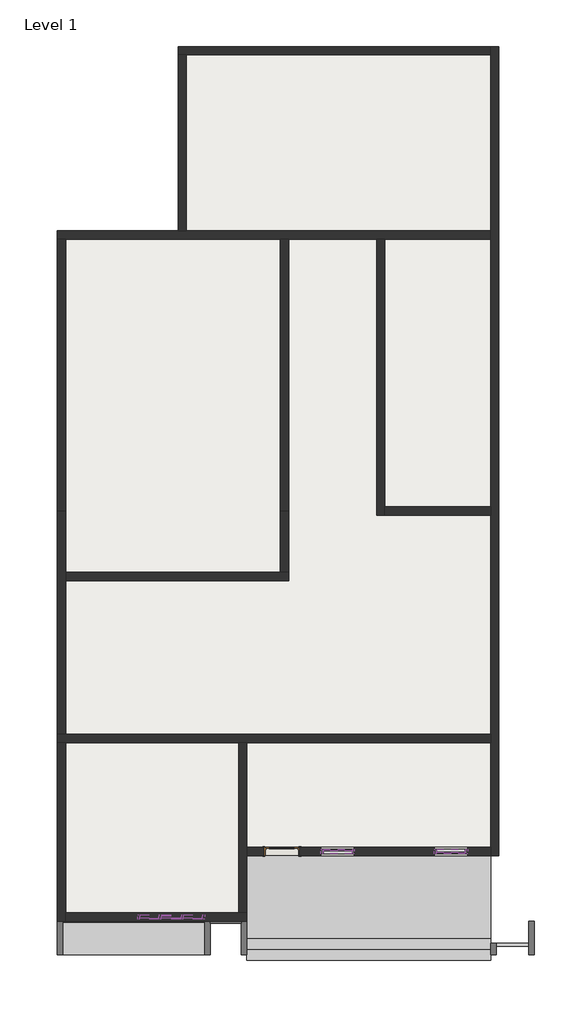
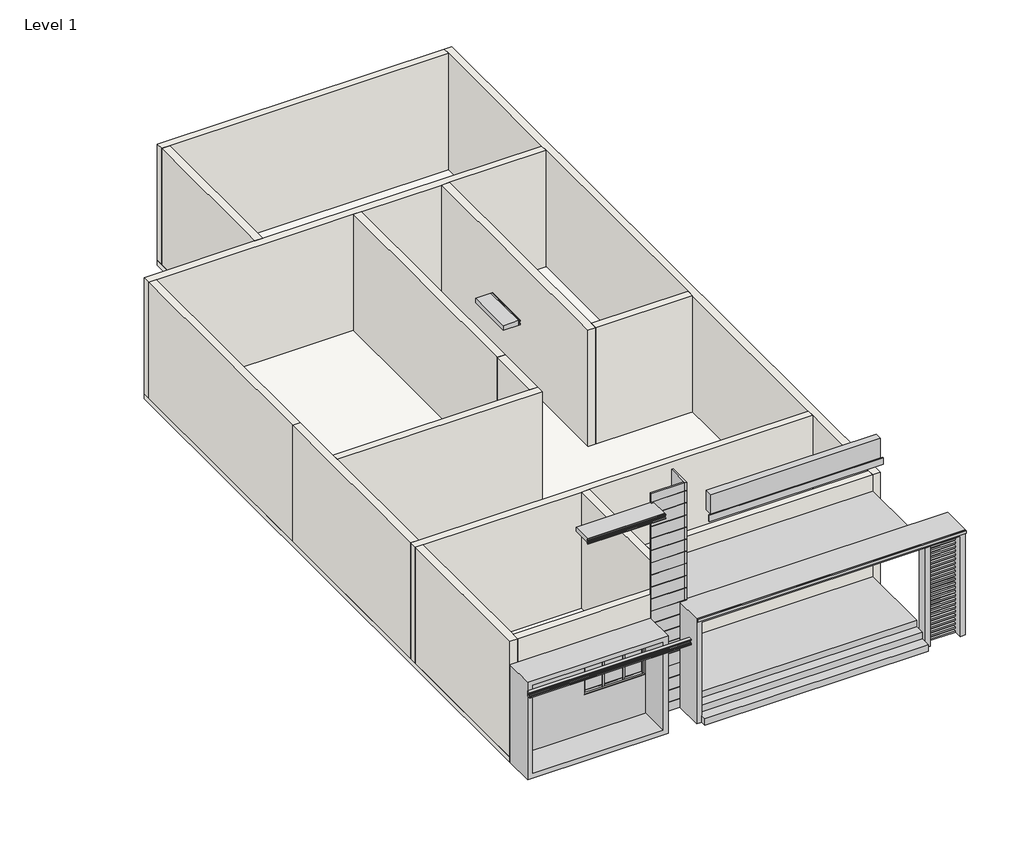
# One storey: 40 members, 16 walls, 11 plates, 2 proxies, 1 door, 1 slab.
"""IFC4 building model written with IfcOpenShell, lengths in millimetres."""

from ifc_helpers import new_model, si_unit, frame, origin, origin_with_axes, place, context, project, spatial, polyline, outline, extrude, faceted_brep, transform, mapped, element, save
from components import generic_models_1_generic_models_1_6f844308, generic_models_2_generic_models_2_638b9eba, door_868ee8a9, member_3578a4a6, member_0b7646a3, member_b3098cb3, member_a980948f, member_ce4f90f2, member_429f6687, member_18a184ad, member_546c81ed, system_panel_glazed_f555cb13, system_panel_glazed_9e7866c3, system_panel_glazed_2ec405e4, system_panel_glazed_c2282f98, system_panel_glazed_db1fed72

model = new_model("IFC4")

# Units and contexts
model_context = context("Model", 3, world=origin())
ifc_project = project(units=[si_unit("LENGTHUNIT", "METRE", prefix="MILLI")], contexts=[model_context])

# Site, building, storey
site = spatial("IfcSite", under=ifc_project)
building = spatial("IfcBuilding", under=site)
storey = spatial("IfcBuildingStorey", under=building, Name="Level 1", Elevation=0.0)

# Proxies
placement = place(None, origin())
generic_models_1_generic_models_1_shape = generic_models_1_generic_models_1_6f844308(model_context)
element("IfcBuildingElementProxy", 1, Name="Generic Models 1 : Generic Models 1", ObjectType="Generic Models 1 : Generic Models 1", at=placement, inside=storey, context=model_context, shape_type="MappedRepresentation", body=[
    mapped(generic_models_1_generic_models_1_shape, transform((0.0, 0.0, 0.0), x_axis=(1.0, 0.0, 0.0), y_axis=(0.0, 1.0, 0.0), z_axis=(0.0, 0.0, 1.0))),
])
generic_models_2_generic_models_2_shape = generic_models_2_generic_models_2_638b9eba(model_context)
element("IfcBuildingElementProxy", 2, Name="Generic Models 2 : Generic Models 2", ObjectType="Generic Models 2 : Generic Models 2", at=placement, inside=storey, context=model_context, shape_type="MappedRepresentation", body=[
    mapped(generic_models_2_generic_models_2_shape, transform((0.0, 0.0, 0.0), x_axis=(1.0, 0.0, 0.0), y_axis=(0.0, 1.0, 0.0), z_axis=(0.0, 0.0, 1.0))),
])

# Door
door_shape = door_868ee8a9(model_context)
element("IfcDoor", 3, ObjectType="Door-Interior-Single-1_Panel-Wood : 36\" x 84\"", at=placement, inside=storey, context=model_context, shape_type="MappedRepresentation", body=[
    mapped(door_shape, transform((-7264.4175664, -12043.8694793, 406.4), x_axis=(-1.0, 0.0, 0.0), y_axis=(0.0, -1.0, 0.0), z_axis=(0.0, 0.0, 1.0))),
])

# Members
member_shape = member_3578a4a6(model_context)
element("IfcMember", 4, ObjectType="Rectangular Mullion : 1.5\" x 2.5\" rectangular", at=placement, inside=storey, context=model_context, shape_type="MappedRepresentation", body=[
    mapped(member_shape, transform((-10560.0675664, -13837.7444793, 2252.1333333), x_axis=(0.0, 0.0, 1.0), y_axis=(0.0, 1.0, 0.0), z_axis=(-1.0, 0.0, 0.0))),
])
element("IfcMember", 5, ObjectType="Rectangular Mullion : 1.5\" x 2.5\" rectangular", at=placement, inside=storey, context=model_context, shape_type="MappedRepresentation", body=[
    mapped(member_shape, transform((-10560.0675664, -13837.7444793, 1735.6666667), x_axis=(0.0, 0.0, 1.0), y_axis=(0.0, 1.0, 0.0), z_axis=(-1.0, 0.0, 0.0))),
])
member_2_shape = member_0b7646a3(model_context)
element("IfcMember", 6, ObjectType="Rectangular Mullion : 2.5\" x 5\" rectangular", at=placement, inside=storey, context=model_context, shape_type="MappedRepresentation", body=[
    mapped(member_2_shape, transform((-11137.9175664, -13837.7444793, 2768.6), x_axis=(0.0, 0.0, 1.0), y_axis=(0.0, 1.0, 0.0), z_axis=(-1.0, 0.0, 0.0))),
])
element("IfcMember", 7, ObjectType="Rectangular Mullion : 2.5\" x 5\" rectangular", at=placement, inside=storey, context=model_context, shape_type="MappedRepresentation", body=[
    mapped(member_2_shape, transform((-9950.4675664, -13837.7444793, 2768.6), x_axis=(0.0, 0.0, 1.0), y_axis=(0.0, 1.0, 0.0), z_axis=(-1.0, 0.0, 0.0))),
])
element("IfcMember", 8, ObjectType="Rectangular Mullion : 2.5\" x 5\" rectangular", at=placement, inside=storey, context=model_context, shape_type="MappedRepresentation", body=[
    mapped(member_2_shape, transform((-9436.1175664, -13837.7444793, 1219.2), x_axis=(0.0, 0.0, -1.0), y_axis=(0.0, 1.0, 0.0), z_axis=(1.0, 0.0, 0.0))),
])
element("IfcMember", 9, ObjectType="Rectangular Mullion : 2.5\" x 5\" rectangular", at=placement, inside=storey, context=model_context, shape_type="MappedRepresentation", body=[
    mapped(member_2_shape, transform((-10623.5675664, -13837.7444793, 1219.2), x_axis=(0.0, 0.0, -1.0), y_axis=(0.0, 1.0, 0.0), z_axis=(1.0, 0.0, 0.0))),
])
member_3_shape = member_b3098cb3(model_context)
element("IfcMember", 10, ObjectType="Rectangular Mullion : 2.5\" x 5\" rectangular", at=placement, inside=storey, context=model_context, shape_type="MappedRepresentation", body=[
    mapped(member_3_shape, transform((-10591.8175664, -13837.7444793, 1219.2), x_axis=(-1.0, 0.0, 0.0), y_axis=(0.0, 1.0, 0.0), z_axis=(0.0, 0.0, -1.0))),
])
element("IfcMember", 11, ObjectType="Rectangular Mullion : 2.5\" x 5\" rectangular", at=placement, inside=storey, context=model_context, shape_type="MappedRepresentation", body=[
    mapped(member_3_shape, transform((-9982.2175664, -13837.7444793, 1219.2), x_axis=(-1.0, 0.0, 0.0), y_axis=(0.0, 1.0, 0.0), z_axis=(0.0, 0.0, -1.0))),
])
member_4_shape = member_a980948f(model_context)
element("IfcMember", 12, ObjectType="Rectangular Mullion : 2.5\" x 5\" rectangular", at=placement, inside=storey, context=model_context, shape_type="MappedRepresentation", body=[
    mapped(member_4_shape, transform((-10013.9675664, -13837.7444793, 1219.2), x_axis=(0.0, 0.0, -1.0), y_axis=(0.0, 1.0, 0.0), z_axis=(1.0, 0.0, 0.0))),
])
element("IfcMember", 13, ObjectType="Rectangular Mullion : 2.5\" x 5\" rectangular", at=placement, inside=storey, context=model_context, shape_type="MappedRepresentation", body=[
    mapped(member_4_shape, transform((-10560.0675664, -13837.7444793, 2768.6), x_axis=(0.0, 0.0, 1.0), y_axis=(0.0, 1.0, 0.0), z_axis=(-1.0, 0.0, 0.0))),
])
element("IfcMember", 14, ObjectType="Rectangular Mullion : 2.5\" x 5\" rectangular", at=placement, inside=storey, context=model_context, shape_type="MappedRepresentation", body=[
    mapped(member_3_shape, transform((-10591.8175664, -13837.7444793, 2252.1333333), x_axis=(-1.0, 0.0, 0.0), y_axis=(0.0, 1.0, 0.0), z_axis=(0.0, 0.0, -1.0))),
])
element("IfcMember", 15, ObjectType="Rectangular Mullion : 2.5\" x 5\" rectangular", at=placement, inside=storey, context=model_context, shape_type="MappedRepresentation", body=[
    mapped(member_3_shape, transform((-9982.2175664, -13837.7444793, 2252.1333333), x_axis=(-1.0, 0.0, 0.0), y_axis=(0.0, 1.0, 0.0), z_axis=(0.0, 0.0, -1.0))),
])
element("IfcMember", 16, ObjectType="Rectangular Mullion : 2.5\" x 5\" rectangular", at=placement, inside=storey, context=model_context, shape_type="MappedRepresentation", body=[
    mapped(member_3_shape, transform((-10591.8175664, -13837.7444793, 1735.6666667), x_axis=(-1.0, 0.0, 0.0), y_axis=(0.0, 1.0, 0.0), z_axis=(0.0, 0.0, -1.0))),
])
element("IfcMember", 17, ObjectType="Rectangular Mullion : 2.5\" x 5\" rectangular", at=placement, inside=storey, context=model_context, shape_type="MappedRepresentation", body=[
    mapped(member_3_shape, transform((-9982.2175664, -13837.7444793, 1735.6666667), x_axis=(-1.0, 0.0, 0.0), y_axis=(0.0, 1.0, 0.0), z_axis=(0.0, 0.0, -1.0))),
])
member_5_shape = member_ce4f90f2(model_context)
element("IfcMember", 18, ObjectType="Rectangular Mullion : 2.5\" x 5\" rectangular", at=placement, inside=storey, context=model_context, shape_type="MappedRepresentation", body=[
    mapped(member_5_shape, transform((-9372.6175664, -13837.7444793, 2768.6), x_axis=(1.0, 0.0, 0.0), y_axis=(0.0, 1.0, 0.0), z_axis=(0.0, 0.0, 1.0))),
])
element("IfcMember", 19, ObjectType="Rectangular Mullion : 2.5\" x 5\" rectangular", at=placement, inside=storey, context=model_context, shape_type="MappedRepresentation", body=[
    mapped(member_5_shape, transform((-11201.4175664, -13837.7444793, 1219.2), x_axis=(-1.0, 0.0, 0.0), y_axis=(0.0, 1.0, 0.0), z_axis=(0.0, 0.0, -1.0))),
])
element("IfcMember", 20, ObjectType="Rectangular Mullion : 2.5\" x 5\" rectangular", at=placement, inside=storey, context=model_context, shape_type="MappedRepresentation", body=[
    mapped(member_5_shape, transform((-11201.4175664, -13837.7444793, 2252.1333333), x_axis=(-1.0, 0.0, 0.0), y_axis=(0.0, 1.0, 0.0), z_axis=(0.0, 0.0, -1.0))),
])
element("IfcMember", 21, ObjectType="Rectangular Mullion : 2.5\" x 5\" rectangular", at=placement, inside=storey, context=model_context, shape_type="MappedRepresentation", body=[
    mapped(member_5_shape, transform((-11201.4175664, -13837.7444793, 1735.6666667), x_axis=(-1.0, 0.0, 0.0), y_axis=(0.0, 1.0, 0.0), z_axis=(0.0, 0.0, -1.0))),
])
element("IfcMember", 22, ObjectType="Rectangular Mullion : 2.5\" x 5\" rectangular", at=placement, inside=storey, context=model_context, shape_type="MappedRepresentation", body=[
    mapped(member_5_shape, transform((-9372.6175664, -13837.7444793, 2252.1333333), x_axis=(1.0, 0.0, 0.0), y_axis=(0.0, 1.0, 0.0), z_axis=(0.0, 0.0, 1.0))),
])
element("IfcMember", 23, ObjectType="Rectangular Mullion : 2.5\" x 5\" rectangular", at=placement, inside=storey, context=model_context, shape_type="MappedRepresentation", body=[
    mapped(member_5_shape, transform((-9372.6175664, -13837.7444793, 1735.6666667), x_axis=(1.0, 0.0, 0.0), y_axis=(0.0, 1.0, 0.0), z_axis=(0.0, 0.0, 1.0))),
])
member_6_shape = member_429f6687(model_context)
element("IfcMember", 24, ObjectType="Rectangular Mullion : 2.5\" x 5\" rectangular", at=placement, inside=storey, context=model_context, shape_type="MappedRepresentation", body=[
    mapped(member_6_shape, transform((-5346.7175664, -12047.0444793, 2768.6), x_axis=(0.0, 0.0, 1.0), y_axis=(0.0, -1.0, 0.0), z_axis=(1.0, 0.0, 0.0))),
])
element("IfcMember", 25, ObjectType="Rectangular Mullion : 2.5\" x 5\" rectangular", at=placement, inside=storey, context=model_context, shape_type="MappedRepresentation", body=[
    mapped(member_6_shape, transform((-3036.5403048, -12047.0444793, 2768.6), x_axis=(0.0, 0.0, 1.0), y_axis=(0.0, 1.0, 0.0), z_axis=(-1.0, 0.0, 0.0))),
])
element("IfcMember", 26, ObjectType="Rectangular Mullion : 2.5\" x 5\" rectangular", at=placement, inside=storey, context=model_context, shape_type="MappedRepresentation", body=[
    mapped(member_6_shape, transform((-6134.1175664, -12047.0444793, 977.8820111), x_axis=(0.0, 0.0, -1.0), y_axis=(0.0, -1.0, 0.0), z_axis=(-1.0, 0.0, 0.0))),
])
element("IfcMember", 27, ObjectType="Rectangular Mullion : 2.5\" x 5\" rectangular", at=placement, inside=storey, context=model_context, shape_type="MappedRepresentation", body=[
    mapped(member_6_shape, transform((-2249.1403048, -12047.0444793, 977.8820111), x_axis=(0.0, 0.0, -1.0), y_axis=(0.0, 1.0, 0.0), z_axis=(1.0, 0.0, 0.0))),
])
member_7_shape = member_18a184ad(model_context)
element("IfcMember", 28, ObjectType="Rectangular Mullion : 2.5\" x 5\" rectangular", at=placement, inside=storey, context=model_context, shape_type="MappedRepresentation", body=[
    mapped(member_7_shape, transform((-5346.7175664, -12047.0444793, 2171.6940037), x_axis=(0.0, 0.0, 1.0), y_axis=(0.0, -1.0, 0.0), z_axis=(1.0, 0.0, 0.0))),
])
element("IfcMember", 29, ObjectType="Rectangular Mullion : 2.5\" x 5\" rectangular", at=placement, inside=storey, context=model_context, shape_type="MappedRepresentation", body=[
    mapped(member_7_shape, transform((-5346.7175664, -12047.0444793, 1574.7880074), x_axis=(0.0, 0.0, 1.0), y_axis=(0.0, -1.0, 0.0), z_axis=(1.0, 0.0, 0.0))),
])
element("IfcMember", 30, ObjectType="Rectangular Mullion : 2.5\" x 5\" rectangular", at=placement, inside=storey, context=model_context, shape_type="MappedRepresentation", body=[
    mapped(member_7_shape, transform((-3036.5403048, -12047.0444793, 2171.6940037), x_axis=(0.0, 0.0, 1.0), y_axis=(0.0, 1.0, 0.0), z_axis=(-1.0, 0.0, 0.0))),
])
element("IfcMember", 31, ObjectType="Rectangular Mullion : 2.5\" x 5\" rectangular", at=placement, inside=storey, context=model_context, shape_type="MappedRepresentation", body=[
    mapped(member_7_shape, transform((-3036.5403048, -12047.0444793, 1574.7880074), x_axis=(0.0, 0.0, 1.0), y_axis=(0.0, 1.0, 0.0), z_axis=(-1.0, 0.0, 0.0))),
])
member_8_shape = member_546c81ed(model_context)
element("IfcMember", 32, ObjectType="Rectangular Mullion : 2.5\" x 5\" rectangular", at=placement, inside=storey, context=model_context, shape_type="MappedRepresentation", body=[
    mapped(member_8_shape, transform((-6197.6175664, -12047.0444793, 2768.6), x_axis=(-1.0, 0.0, 0.0), y_axis=(0.0, -1.0, 0.0), z_axis=(0.0, 0.0, 1.0))),
])
element("IfcMember", 33, ObjectType="Rectangular Mullion : 2.5\" x 5\" rectangular", at=placement, inside=storey, context=model_context, shape_type="MappedRepresentation", body=[
    mapped(member_8_shape, transform((-2185.6403048, -12047.0444793, 2768.6), x_axis=(1.0, 0.0, 0.0), y_axis=(0.0, 1.0, 0.0), z_axis=(0.0, 0.0, 1.0))),
])
element("IfcMember", 34, ObjectType="Rectangular Mullion : 2.5\" x 5\" rectangular", at=placement, inside=storey, context=model_context, shape_type="MappedRepresentation", body=[
    mapped(member_8_shape, transform((-5283.2175664, -12047.0444793, 977.8820111), x_axis=(1.0, 0.0, 0.0), y_axis=(0.0, -1.0, 0.0), z_axis=(0.0, 0.0, -1.0))),
])
element("IfcMember", 35, ObjectType="Rectangular Mullion : 2.5\" x 5\" rectangular", at=placement, inside=storey, context=model_context, shape_type="MappedRepresentation", body=[
    mapped(member_8_shape, transform((-3100.0403048, -12047.0444793, 977.8820111), x_axis=(-1.0, 0.0, 0.0), y_axis=(0.0, 1.0, 0.0), z_axis=(0.0, 0.0, -1.0))),
])
element("IfcMember", 36, ObjectType="Rectangular Mullion : 2.5\" x 5\" rectangular", at=placement, inside=storey, context=model_context, shape_type="MappedRepresentation", body=[
    mapped(member_8_shape, transform((-5283.2175664, -12047.0444793, 2171.6940037), x_axis=(1.0, 0.0, 0.0), y_axis=(0.0, -1.0, 0.0), z_axis=(0.0, 0.0, -1.0))),
])
element("IfcMember", 37, ObjectType="Rectangular Mullion : 2.5\" x 5\" rectangular", at=placement, inside=storey, context=model_context, shape_type="MappedRepresentation", body=[
    mapped(member_8_shape, transform((-3100.0403048, -12047.0444793, 2171.6940037), x_axis=(-1.0, 0.0, 0.0), y_axis=(0.0, 1.0, 0.0), z_axis=(0.0, 0.0, -1.0))),
])
element("IfcMember", 38, ObjectType="Rectangular Mullion : 2.5\" x 5\" rectangular", at=placement, inside=storey, context=model_context, shape_type="MappedRepresentation", body=[
    mapped(member_8_shape, transform((-5283.2175664, -12047.0444793, 1574.7880074), x_axis=(1.0, 0.0, 0.0), y_axis=(0.0, -1.0, 0.0), z_axis=(0.0, 0.0, -1.0))),
])
element("IfcMember", 39, ObjectType="Rectangular Mullion : 2.5\" x 5\" rectangular", at=placement, inside=storey, context=model_context, shape_type="MappedRepresentation", body=[
    mapped(member_8_shape, transform((-3100.0403048, -12047.0444793, 1574.7880074), x_axis=(-1.0, 0.0, 0.0), y_axis=(0.0, 1.0, 0.0), z_axis=(0.0, 0.0, -1.0))),
])
element("IfcMember", 40, ObjectType="Rectangular Mullion : 2.5\" x 5\" rectangular", at=placement, inside=storey, context=model_context, shape_type="MappedRepresentation", body=[
    mapped(member_8_shape, transform((-6197.6175664, -12047.0444793, 2171.6940037), x_axis=(-1.0, 0.0, 0.0), y_axis=(0.0, -1.0, 0.0), z_axis=(0.0, 0.0, 1.0))),
])
element("IfcMember", 41, ObjectType="Rectangular Mullion : 2.5\" x 5\" rectangular", at=placement, inside=storey, context=model_context, shape_type="MappedRepresentation", body=[
    mapped(member_8_shape, transform((-2185.6403048, -12047.0444793, 2171.6940037), x_axis=(1.0, 0.0, 0.0), y_axis=(0.0, 1.0, 0.0), z_axis=(0.0, 0.0, 1.0))),
])
element("IfcMember", 42, ObjectType="Rectangular Mullion : 2.5\" x 5\" rectangular", at=placement, inside=storey, context=model_context, shape_type="MappedRepresentation", body=[
    mapped(member_8_shape, transform((-6197.6175664, -12047.0444793, 1574.7880074), x_axis=(-1.0, 0.0, 0.0), y_axis=(0.0, -1.0, 0.0), z_axis=(0.0, 0.0, 1.0))),
])
element("IfcMember", 43, ObjectType="Rectangular Mullion : 2.5\" x 5\" rectangular", at=placement, inside=storey, context=model_context, shape_type="MappedRepresentation", body=[
    mapped(member_8_shape, transform((-2185.6403048, -12047.0444793, 1574.7880074), x_axis=(1.0, 0.0, 0.0), y_axis=(0.0, 1.0, 0.0), z_axis=(0.0, 0.0, 1.0))),
])

# Plates
system_panel_glazed_shape = system_panel_glazed_f555cb13(model_context)
element("IfcPlate", 44, ObjectType="System Panel : Glazed", at=placement, inside=storey, context=model_context, shape_type="MappedRepresentation", body=[
    mapped(system_panel_glazed_shape, transform((-9693.2925664, -13837.7444793, 1282.7), x_axis=(-1.0, 0.0, 0.0), y_axis=(0.0, -1.0, 0.0), z_axis=(0.0, 0.0, 1.0))),
])
element("IfcPlate", 45, ObjectType="System Panel : Glazed", at=placement, inside=storey, context=model_context, shape_type="MappedRepresentation", body=[
    mapped(system_panel_glazed_shape, transform((-10880.7425664, -13837.7444793, 1282.7), x_axis=(-1.0, 0.0, 0.0), y_axis=(0.0, -1.0, 0.0), z_axis=(0.0, 0.0, 1.0))),
])
system_panel_glazed_2_shape = system_panel_glazed_9e7866c3(model_context)
element("IfcPlate", 46, ObjectType="System Panel : Glazed", at=placement, inside=storey, context=model_context, shape_type="MappedRepresentation", body=[
    mapped(system_panel_glazed_2_shape, transform((-10287.0175664, -13837.7444793, 1282.7), x_axis=(-1.0, 0.0, 0.0), y_axis=(0.0, -1.0, 0.0), z_axis=(0.0, 0.0, 1.0))),
])
element("IfcPlate", 47, ObjectType="System Panel : Glazed", at=placement, inside=storey, context=model_context, shape_type="MappedRepresentation", body=[
    mapped(system_panel_glazed_2_shape, transform((-10287.0175664, -13837.7444793, 2271.1833333), x_axis=(-1.0, 0.0, 0.0), y_axis=(0.0, -1.0, 0.0), z_axis=(0.0, 0.0, 1.0))),
])
system_panel_glazed_3_shape = system_panel_glazed_2ec405e4(model_context)
element("IfcPlate", 48, ObjectType="System Panel : Glazed", at=placement, inside=storey, context=model_context, shape_type="MappedRepresentation", body=[
    mapped(system_panel_glazed_3_shape, transform((-10287.0175664, -13837.7444793, 1754.7166667), x_axis=(-1.0, 0.0, 0.0), y_axis=(0.0, -1.0, 0.0), z_axis=(0.0, 0.0, 1.0))),
])
system_panel_glazed_4_shape = system_panel_glazed_c2282f98(model_context)
element("IfcPlate", 49, ObjectType="System Panel : Glazed", at=placement, inside=storey, context=model_context, shape_type="MappedRepresentation", body=[
    mapped(system_panel_glazed_4_shape, transform((-5740.4175664, -12047.0444793, 1041.3820111), x_axis=(1.0, 0.0, 0.0), y_axis=(0.0, 1.0, 0.0), z_axis=(0.0, 0.0, 1.0))),
])
element("IfcPlate", 50, ObjectType="System Panel : Glazed", at=placement, inside=storey, context=model_context, shape_type="MappedRepresentation", body=[
    mapped(system_panel_glazed_4_shape, transform((-2642.8403048, -12047.0444793, 1041.3820111), x_axis=(-1.0, 0.0, 0.0), y_axis=(0.0, -1.0, 0.0), z_axis=(0.0, 0.0, 1.0))),
])
element("IfcPlate", 51, ObjectType="System Panel : Glazed", at=placement, inside=storey, context=model_context, shape_type="MappedRepresentation", body=[
    mapped(system_panel_glazed_4_shape, transform((-5740.4175664, -12047.0444793, 2203.4440037), x_axis=(1.0, 0.0, 0.0), y_axis=(0.0, 1.0, 0.0), z_axis=(0.0, 0.0, 1.0))),
])
element("IfcPlate", 52, ObjectType="System Panel : Glazed", at=placement, inside=storey, context=model_context, shape_type="MappedRepresentation", body=[
    mapped(system_panel_glazed_4_shape, transform((-2642.8403048, -12047.0444793, 2203.4440037), x_axis=(-1.0, 0.0, 0.0), y_axis=(0.0, -1.0, 0.0), z_axis=(0.0, 0.0, 1.0))),
])
system_panel_glazed_5_shape = system_panel_glazed_db1fed72(model_context)
element("IfcPlate", 53, ObjectType="System Panel : Glazed", at=placement, inside=storey, context=model_context, shape_type="MappedRepresentation", body=[
    mapped(system_panel_glazed_5_shape, transform((-5740.4175664, -12047.0444793, 1606.5380074), x_axis=(1.0, 0.0, 0.0), y_axis=(0.0, 1.0, 0.0), z_axis=(0.0, 0.0, 1.0))),
])
element("IfcPlate", 54, ObjectType="System Panel : Glazed", at=placement, inside=storey, context=model_context, shape_type="MappedRepresentation", body=[
    mapped(system_panel_glazed_5_shape, transform((-2642.8403048, -12047.0444793, 1606.5380074), x_axis=(-1.0, 0.0, 0.0), y_axis=(0.0, -1.0, 0.0), z_axis=(0.0, 0.0, 1.0))),
])

# Slab
element("IfcSlab", 55, ObjectType="ground floor 6\"", at=placement, inside=storey, context=model_context, shape_type="SweptSolid", body=[
    extrude(outline(polyline([(-10097.7403048, 9936.6555207), (-1334.7403048, 9936.6555207), (-1334.7403048, -12161.3444793), (-8216.9175664, -12161.3444793), (-8216.9175664, -13952.0444793), (-13398.5175664, -13952.0444793), (-13398.5175664, 4907.4555207), (-10097.7403048, 4907.4555207), (-10097.7403048, 9936.6555207)])), frame((0.0, 0.0, -152.4), z_axis=(0.0, 0.0, 1.0), x_axis=(1.0, 0.0, 0.0)), (0.0, 0.0, 1.0), 152.4),
])

# Walls
element("IfcWall", 56, ObjectType="9\" wall", at=placement, inside=storey, context=model_context, shape_type="Brep", body=[
    faceted_brep([(-10097.7403048, 9708.0555207, 0.0), (-9869.1403048, 9708.0555207, 0.0), (-1563.3403048, 9708.0555207, 0.0), (-1563.3403048, 9708.0555207, 3657.6), (-9869.1403048, 9708.0555207, 3657.6), (-10097.7403048, 9708.0555207, 3657.6), (-10097.7403048, 9936.6555207, 0.0), (-10097.7403048, 9936.6555207, 3657.6), (-1563.3403048, 9936.6555207, 3657.6), (-1563.3403048, 9936.6555207, 0.0)], [[[0, 1, 2, 3, 4, 5]], [[6, 7, 8, 9]], [[2, 1, 0, 6, 9]], [[5, 4, 3, 8, 7]], [[0, 5, 7, 6]], [[3, 2, 9, 8]]]),
])
element("IfcWall", 57, ObjectType="9\" wall", at=placement, inside=storey, context=model_context, shape_type="SweptSolid", body=[
    extrude(outline(polyline([(-9869.1403048, 9708.0555207), (-9869.1403048, 4907.4555207), (-10097.7403048, 4907.4555207), (-10097.7403048, 9708.0555207), (-9869.1403048, 9708.0555207)])), origin_with_axes(), (0.0, 0.0, 1.0), 3657.6),
])
element("IfcWall", 58, ObjectType="9\" wall", at=placement, inside=storey, context=model_context, shape_type="Brep", body=[
    faceted_brep([(-1563.3403048, 4907.4555207, 0.0), (-9869.1403048, 4907.4555207, 0.0), (-10097.7403048, 4907.4555207, 0.0), (-13398.5175664, 4907.4555207, 0.0), (-13398.5175664, 4907.4555207, 3657.6), (-10097.7403048, 4907.4555207, 3657.6), (-9869.1403048, 4907.4555207, 3657.6), (-1563.3403048, 4907.4555207, 3657.6), (-1563.3403048, 4678.8555207, 0.0), (-1563.3403048, 4678.8555207, 3657.6), (-4446.2403048, 4678.8555207, 3657.6), (-4674.8403048, 4678.8555207, 3657.6), (-7073.9175664, 4678.8555207, 3657.6), (-7302.5175664, 4678.8555207, 3657.6), (-13169.9175664, 4678.8555207, 3657.6), (-13398.5175664, 4678.8555207, 3657.6), (-13398.5175664, 4678.8555207, 0.0), (-13169.9175664, 4678.8555207, 0.0), (-7302.5175664, 4678.8555207, 0.0), (-7073.9175664, 4678.8555207, 0.0), (-4674.8403048, 4678.8555207, 0.0), (-4446.2403048, 4678.8555207, 0.0)], [[[0, 1, 2, 3, 4, 5, 6, 7]], [[8, 9, 10, 11, 12, 13, 14, 15, 16, 17, 18, 19, 20, 21]], [[3, 2, 1, 0, 8, 21, 20, 19, 18, 17, 16]], [[7, 6, 5, 4, 15, 14, 13, 12, 11, 10, 9]], [[4, 3, 16, 15]], [[0, 7, 9, 8]]]),
])
element("IfcWall", 59, ObjectType="9\" wall", at=placement, inside=storey, context=model_context, shape_type="Brep", body=[
    faceted_brep([(-1563.3403048, 9936.6555207, 0.0), (-1563.3403048, 9708.0555207, 0.0), (-1563.3403048, 4907.4555207, 0.0), (-1563.3403048, 4678.8555207, 0.0), (-1563.3403048, -2636.3444793, 0.0), (-1563.3403048, -2864.9444793, 0.0), (-1563.3403048, -8846.6444793, 0.0), (-1563.3403048, -9075.2444793, 0.0), (-1563.3403048, -11932.7444793, 0.0), (-1563.3403048, -12161.3444793, 0.0), (-1563.3403048, -12161.3444793, 3657.6), (-1563.3403048, -11932.7444793, 3657.6), (-1563.3403048, -9075.2444793, 3657.6), (-1563.3403048, -8846.6444793, 3657.6), (-1563.3403048, -2864.9444793, 3657.6), (-1563.3403048, -2636.3444793, 3657.6), (-1563.3403048, 4678.8555207, 3657.6), (-1563.3403048, 4907.4555207, 3657.6), (-1563.3403048, 9708.0555207, 3657.6), (-1563.3403048, 9936.6555207, 3657.6), (-1334.7403048, 9936.6555207, 0.0), (-1334.7403048, 9936.6555207, 3657.6), (-1334.7403048, -12161.3444793, 3657.6), (-1334.7403048, -12161.3444793, 0.0)], [[[0, 1, 2, 3, 4, 5, 6, 7, 8, 9, 10, 11, 12, 13, 14, 15, 16, 17, 18, 19]], [[20, 21, 22, 23]], [[9, 8, 7, 6, 5, 4, 3, 2, 1, 0, 20, 23]], [[19, 18, 17, 16, 15, 14, 13, 12, 11, 10, 22, 21]], [[0, 19, 21, 20]], [[10, 9, 23, 22]]]),
])
element("IfcWall", 60, ObjectType="9\" wall", at=placement, inside=storey, context=model_context, shape_type="SweptSolid", body=[
    extrude(outline(polyline([(-13169.9175664, 4678.8555207), (-13169.9175664, -2750.6444793), (-13398.5175664, -2750.6444793), (-13398.5175664, 4678.8555207), (-13169.9175664, 4678.8555207)])), origin_with_axes(), (0.0, 0.0, 1.0), 3657.6),
])
element("IfcWall", 61, ObjectType="9\" wall", at=placement, inside=storey, context=model_context, shape_type="SweptSolid", body=[
    extrude(outline(polyline([(-7302.5175664, -2750.6444793), (-7302.5175664, 4678.8555207), (-7073.9175664, 4678.8555207), (-7073.9175664, -2750.6444793), (-7302.5175664, -2750.6444793)])), origin_with_axes(), (0.0, 0.0, 1.0), 3657.6),
])
element("IfcWall", 62, ObjectType="9\" wall", at=placement, inside=storey, context=model_context, shape_type="Brep", body=[
    faceted_brep([(-4674.8403048, 4678.8555207, 0.0), (-4674.8403048, -2864.9444793, 0.0), (-4674.8403048, -2864.9444793, 3657.6), (-4674.8403048, 4678.8555207, 3657.6), (-4446.2403048, 4678.8555207, 0.0), (-4446.2403048, 4678.8555207, 3657.6), (-4446.2403048, -2636.3444793, 3657.6), (-4446.2403048, -2864.9444793, 3657.6), (-4446.2403048, -2864.9444793, 0.0), (-4446.2403048, -2636.3444793, 0.0)], [[[0, 1, 2, 3]], [[4, 5, 6, 7, 8, 9]], [[1, 0, 4, 9, 8]], [[3, 2, 7, 6, 5]], [[0, 3, 5, 4]], [[2, 1, 8, 7]]]),
])
element("IfcWall", 63, ObjectType="9\" wall", at=placement, inside=storey, context=model_context, shape_type="SweptSolid", body=[
    extrude(outline(polyline([(-1563.3403048, -2864.9444793), (-4446.2403048, -2864.9444793), (-4446.2403048, -2636.3444793), (-1563.3403048, -2636.3444793), (-1563.3403048, -2864.9444793)])), origin_with_axes(), (0.0, 0.0, 1.0), 3657.6),
])
element("IfcWall", 64, ObjectType="9\" wall", at=placement, inside=storey, context=model_context, shape_type="Brep", body=[
    faceted_brep([(-1563.3403048, -8846.6444793, 0.0), (-13169.9175664, -8846.6444793, 0.0), (-13398.5175664, -8846.6444793, 0.0), (-13398.5175664, -8846.6444793, 3657.6), (-13169.9175664, -8846.6444793, 3657.6), (-1563.3403048, -8846.6444793, 3657.6), (-1563.3403048, -9075.2444793, 0.0), (-1563.3403048, -9075.2444793, 3657.6), (-8216.9175664, -9075.2444793, 3657.6), (-8445.5175664, -9075.2444793, 3657.6), (-13169.9175664, -9075.2444793, 3657.6), (-13398.5175664, -9075.2444793, 3657.6), (-13398.5175664, -9075.2444793, 0.0), (-13169.9175664, -9075.2444793, 0.0), (-8445.5175664, -9075.2444793, 0.0), (-8216.9175664, -9075.2444793, 0.0)], [[[0, 1, 2, 3, 4, 5]], [[6, 7, 8, 9, 10, 11, 12, 13, 14, 15]], [[2, 1, 0, 6, 15, 14, 13, 12]], [[5, 4, 3, 11, 10, 9, 8, 7]], [[0, 5, 7, 6]], [[3, 2, 12, 11]]]),
])
element("IfcWall", 65, ObjectType="9\" wall", at=placement, inside=storey, context=model_context, shape_type="Brep", body=[
    faceted_brep([(-13169.9175664, -8846.6444793, 0.0), (-13169.9175664, -4655.6444793, 0.0), (-13169.9175664, -4427.0444793, 0.0), (-13169.9175664, -2750.6444793, 0.0), (-13169.9175664, -2750.6444793, 3657.6), (-13169.9175664, -4427.0444793, 3657.6), (-13169.9175664, -4655.6444793, 3657.6), (-13169.9175664, -8846.6444793, 3657.6), (-13398.5175664, -8846.6444793, 0.0), (-13398.5175664, -8846.6444793, 3657.6), (-13398.5175664, -2750.6444793, 3657.6), (-13398.5175664, -2750.6444793, 0.0)], [[[0, 1, 2, 3, 4, 5, 6, 7]], [[8, 9, 10, 11]], [[3, 2, 1, 0, 8, 11]], [[4, 3, 11, 10]], [[7, 6, 5, 4, 10, 9]], [[0, 7, 9, 8]]]),
])
element("IfcWall", 66, ObjectType="9\" wall", at=placement, inside=storey, context=model_context, shape_type="Brep", body=[
    faceted_brep([(-13169.9175664, -4655.6444793, 0.0), (-7073.9175664, -4655.6444793, 0.0), (-7073.9175664, -4655.6444793, 3657.6), (-13169.9175664, -4655.6444793, 3657.6), (-13169.9175664, -4427.0444793, 0.0), (-13169.9175664, -4427.0444793, 3657.6), (-7302.5175664, -4427.0444793, 3657.6), (-7073.9175664, -4427.0444793, 3657.6), (-7073.9175664, -4427.0444793, 0.0), (-7302.5175664, -4427.0444793, 0.0)], [[[0, 1, 2, 3]], [[4, 5, 6, 7, 8, 9]], [[1, 0, 4, 9, 8]], [[3, 2, 7, 6, 5]], [[0, 3, 5, 4]], [[2, 1, 8, 7]]]),
])
element("IfcWall", 67, ObjectType="9\" wall", at=placement, inside=storey, context=model_context, shape_type="SweptSolid", body=[
    extrude(outline(polyline([(-7073.9175664, -2750.6444793), (-7073.9175664, -4427.0444793), (-7302.5175664, -4427.0444793), (-7302.5175664, -2750.6444793), (-7073.9175664, -2750.6444793)])), origin_with_axes(), (0.0, 0.0, 1.0), 3657.6),
])
element("IfcWall", 68, ObjectType="9\" wall", at=placement, inside=storey, context=model_context, shape_type="Brep", body=[
    faceted_brep([(-13398.5175664, -9075.2444793, 0.0), (-13398.5175664, -13952.0444793, 0.0), (-13398.5175664, -13952.0444793, 3657.6), (-13398.5175664, -9075.2444793, 3657.6), (-13169.9175664, -9075.2444793, 0.0), (-13169.9175664, -9075.2444793, 3657.6), (-13169.9175664, -13723.4444793, 3657.6), (-13169.9175664, -13952.0444793, 3657.6), (-13169.9175664, -13952.0444793, 0.0), (-13169.9175664, -13723.4444793, 0.0)], [[[0, 1, 2, 3]], [[4, 5, 6, 7, 8, 9]], [[1, 0, 4, 9, 8]], [[3, 2, 7, 6, 5]], [[0, 3, 5, 4]], [[2, 1, 8, 7]]]),
])
element("IfcWall", 69, ObjectType="9\" wall", at=placement, inside=storey, context=model_context, shape_type="Brep", body=[
    faceted_brep([(-13169.9175664, -13952.0444793, 0.0), (-8216.9175664, -13952.0444793, 0.0), (-8216.9175664, -13952.0444793, 3657.6), (-13169.9175664, -13952.0444793, 3657.6), (-9372.6175664, -13952.0444793, 2768.6), (-9372.6175664, -13952.0444793, 1219.2), (-11201.4175664, -13952.0444793, 1219.2), (-11201.4175664, -13952.0444793, 2768.6), (-8216.9175664, -13723.4444793, 0.0), (-8445.5175664, -13723.4444793, 0.0), (-13169.9175664, -13723.4444793, 0.0), (-13169.9175664, -13723.4444793, 3657.6), (-8445.5175664, -13723.4444793, 3657.6), (-8216.9175664, -13723.4444793, 3657.6), (-9372.6175664, -13723.4444793, 1219.2), (-9372.6175664, -13723.4444793, 2768.6), (-11201.4175664, -13723.4444793, 2768.6), (-11201.4175664, -13723.4444793, 1219.2)], [[[0, 1, 2, 3], [4, 5, 6, 7]], [[8, 9, 10, 11, 12, 13], [14, 15, 16, 17]], [[1, 0, 10, 9, 8]], [[3, 2, 13, 12, 11]], [[0, 3, 11, 10]], [[2, 1, 8, 13]], [[14, 5, 4, 15]], [[15, 4, 7, 16]], [[16, 7, 6, 17]], [[5, 14, 17, 6]]]),
])
element("IfcWall", 70, ObjectType="9\" wall", at=placement, inside=storey, context=model_context, shape_type="Brep", body=[
    faceted_brep([(-8216.9175664, -13723.4444793, 0.0), (-8216.9175664, -12161.3444793, 0.0), (-8216.9175664, -11932.7444793, 0.0), (-8216.9175664, -9075.2444793, 0.0), (-8216.9175664, -9075.2444793, 3657.6), (-8216.9175664, -11932.7444793, 3657.6), (-8216.9175664, -12161.3444793, 3657.6), (-8216.9175664, -13723.4444793, 3657.6), (-8445.5175664, -13723.4444793, 0.0), (-8445.5175664, -13723.4444793, 3657.6), (-8445.5175664, -9075.2444793, 3657.6), (-8445.5175664, -9075.2444793, 0.0)], [[[0, 1, 2, 3, 4, 5, 6, 7]], [[8, 9, 10, 11]], [[3, 2, 1, 0, 8, 11]], [[7, 6, 5, 4, 10, 9]], [[0, 7, 9, 8]], [[4, 3, 11, 10]]]),
])
element("IfcWall", 71, ObjectType="9\" wall", at=placement, inside=storey, context=model_context, shape_type="SweptSolid", body=[
    extrude(outline(polyline([(0.0, -8216.9175664), (0.0, -1563.3403048), (3657.6, -1563.3403048), (3657.6, -8216.9175664), (0.0, -8216.9175664)]), holes=[polyline([(406.4, -7747.0175664), (2565.4, -7747.0175664), (2565.4, -6781.8175664), (406.4, -6781.8175664), (406.4, -7747.0175664)]), polyline([(977.8820111, -6197.6175664), (2768.6, -6197.6175664), (2768.6, -5283.2175664), (977.8820111, -5283.2175664), (977.8820111, -6197.6175664)]), polyline([(2768.6, -2185.6403048), (977.8820111, -2185.6403048), (977.8820111, -3100.0403048), (2768.6, -3100.0403048), (2768.6, -2185.6403048)])]), frame((0.0, -12161.3444793, 0.0), z_axis=(0.0, 1.0, 0.0), x_axis=(0.0, 0.0, 1.0)), (0.0, 0.0, 1.0), 228.6),
])

save(model, "model.ifc")

# Revit data of these elements
# Type "Door-Interior-Single-1_Panel-Wood : 36\" x 84\""
#   Type Mark = "8"
#   Assembly Code = "C1020300"
#   Analytic Construction = "Wooden"
#   Top Rail = 0' - 4 11/16"
#   Thickness = 0' - 1 3/8"
#   Thermal Resistance (R) = 2.5876 (h·ft²·°F)/BTU
#   Swing Angle [instance default] = 90.00°
#   Stiles = 0' - 4 3/4"
#   Rough Width = 3' - 2"
#   Rough Height = 7' - 1"
#   Height = 7' - 0"
#   Width = 3' - 0"
#   Heat Transfer Coefficient (U) = 0.3865 BTU/(h·ft²·°F)
#   Bottom Rail = 0' - 9 1/8"
#   Trim Material = Cherry
#   Panel Material = Cherry
#   Frame Material = Cherry
#   Door Handle Material = Aluminum
#   Visual Light Transmittance = 0
#   Solar Heat Gain Coefficient = 0
#   Wall Closure = (empty or 0)
#   Function = (empty or 0)
# Type "Rectangular Mullion : 1.5\" x 2.5\" rectangular"
#   built-in parameter 1007304 = 0.208333 (stored number, unit not read)
#   built-in parameter 1007301 = 0.0625 (stored number, unit not read)
#   built-in parameter 1007300 = 0.0625 (stored number, unit not read)
# Type "Rectangular Mullion : 2.5\" x 5\" rectangular"
#   built-in parameter 1007304 = 0.416667 (stored number, unit not read)
#   built-in parameter 1007301 = 0.104167 (stored number, unit not read)
#   built-in parameter 1007300 = 0.104167 (stored number, unit not read)
# Type "System Panel : Glazed"
#   Construction Type Id = "GSP4R"
#   Analytic Construction = "1/8 in Pilkington single glazing"
#   Visual Light Transmittance = 0.9
#   Solar Heat Gain Coefficient = 0.86
#   Heat Transfer Coefficient (U) = 1.18115 BTU/(h·ft²·°F)
#   Define Thermal Properties by = 1
# Type "ground floor 6\""
#   Assembly Code = "B1010"
#   Function = 0
# Type "9\" wall"
#   Assembly Code = "B2010"
# Element 1 (IfcBuildingElementProxy, "Generic Models 1 : Generic Models 1")
#   Phase Created = New Construction
#   Materials on its faces: "Laminate, Ivory, Matte"
# Element 2 (IfcBuildingElementProxy, "Generic Models 2 : Generic Models 2")
#   Phase Created = New Construction
#   Materials on its faces: "Gypsum Wall Board", "Damp-proofing", "Laminate, Ivory, Matte", "window wall", "wood balcony"
# Element 3 (IfcDoor, "Door-Interior-Single-1_Panel-Wood : 36\" x 84\"")
#   Swing Angle = 90.00°
#   Phase Created = New Construction
#   Materials on its faces: "Cherry", "Aluminum"
# Elements 4, 5 (IfcMember, "Rectangular Mullion : 1.5\" x 2.5\" rectangular")
#   Phase Created = New Construction
#   Materials on its faces: "Aluminum"
# Elements 6, 7, 8, 9, 10, 11, 12, 13, 14, 15, 16, 17, 18, 19, 20, 21, 22, 23, 24, 25, 26, 27, 28, 29, 30, 31, 32, 33, 34, 35, 36, 37, 38, 39, 40, 41, 42, 43 (IfcMember, "Rectangular Mullion : 2.5\" x 5\" rectangular")
#   Phase Created = New Construction
# Elements 44, 45, 46, 47, 48, 49, 50, 51, 52, 53, 54 (IfcPlate, "System Panel : Glazed")
#   Phase Created = New Construction
#   Materials on its faces: "Glass"
# Element 55 (IfcSlab, "ground floor 6\"")
#   built-in parameter 1001955 = 3.14159 (stored number, unit not read)
#   Height Offset From Level = 0' - 0"
#   Phase Created = New Construction
# Elements 56, 57, 58, 59, 60, 61, 62, 63, 64, 65, 66, 67, 68, 69, 70, 71 (IfcWall, "9\" wall")
#   Top Offset = 0' - 0"
#   Base Offset = 0' - 0"
#   wall height = 12' - 0"
#   Phase Created = New Construction
#   Base Constraint = Level 1
#   Top Constraint = Level 2
# Materials
#   "Cherry": class "Wood", colour RGB 226 177 128, transparency 0, Description = "Prunus Serotina", Cost = 0
#   "Aluminum": class "Metal", colour RGB 247 247 247, transparency 0, Description = "Aluminum 6061", Cost = 0
#   "Laminate, Ivory, Matte": class "Plastic", colour RGB 247 247 239, transparency 0, Description = "Plastic Laminate - Ivory, Matte", Cost = 0
#   "Gypsum Wall Board": class "Generic", colour RGB 127 127 127, transparency 0, Description = "Gypsum Wall Board", Cost = 0
#   "Damp-proofing": class "Generic", colour RGB 127 127 127, transparency 0, Description = "Damp-proofing", Cost = 0
#   "window wall": class "Generic", colour RGB 120 120 120, transparency 0, Cost = 0
#   "wood balcony": class "Generic", colour RGB 120 120 120, transparency 0, Cost = 0
#   "Glass": class "Glass", colour RGB 0 128 192, transparency 0.75, Description = "Soda Lime Glass", Cost = 0
